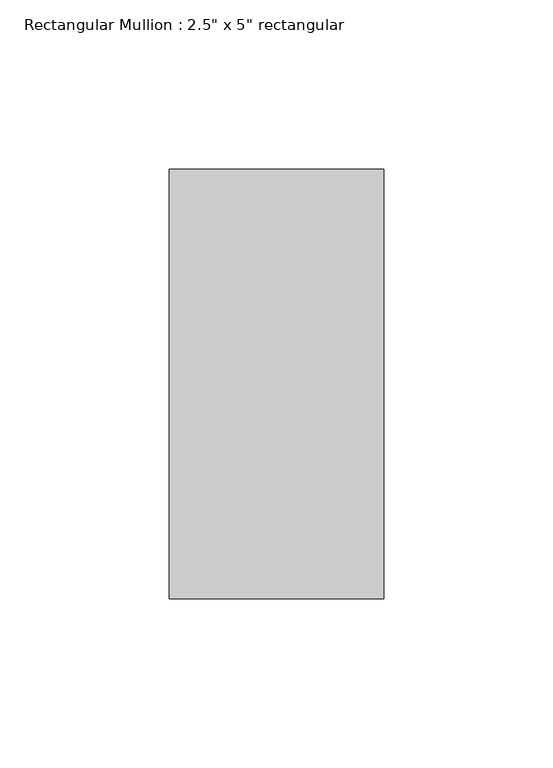
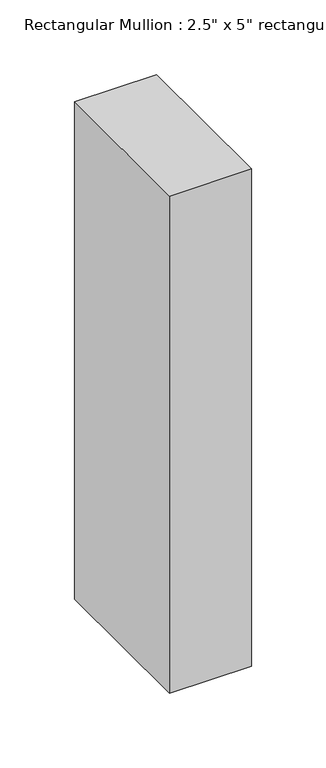
"""IFC4 building model written with IfcOpenShell, lengths in millimetres: member geometry."""

from ifc_helpers import new_model, si_unit, frame, origin, place, context, project, spatial, polyline, outline, extrude, source, transform, mapped, element, save


def member_90c805a2(model_context):
    return source(origin(), model_context, "Body", "SweptSolid", [
        extrude(outline(polyline([(31.75, 63.5), (31.75, -63.5), (-31.75, -63.5), (-31.75, 63.5), (31.75, 63.5)])), frame((0.0, 0.0, -406.4), z_axis=(0.0, 0.0, 1.0), x_axis=(1.0, 0.0, 0.0)), (0.0, 0.0, 1.0), 406.4),
    ])


if __name__ == "__main__":
    model = new_model("IFC4")
    model_context = context("Model", 3, world=origin())
    ifc_project = project(units=[si_unit("LENGTHUNIT", "METRE", prefix="MILLI")], contexts=[model_context])
    site = spatial("IfcSite", under=ifc_project)
    building = spatial("IfcBuilding", under=site)
    placement = place(None, origin())
    member_shape = member_90c805a2(model_context)
    element("IfcMember", 1, ObjectType="Rectangular Mullion : 2.5\" x 5\" rectangular", at=placement, inside=building, context=model_context, shape_type="MappedRepresentation", body=[
        mapped(member_shape, transform((0.0, 0.0, 0.0), x_axis=(1.0, 0.0, 0.0), y_axis=(0.0, 1.0, 0.0), z_axis=(0.0, 0.0, 1.0))),
    ])
    save(model, "model.ifc")

# Revit data of these elements
# Type "Rectangular Mullion : 2.5\" x 5\" rectangular"
#   built-in parameter 1007304 = 0.416667 (stored number, unit not read)
#   built-in parameter 1007301 = 0.104167 (stored number, unit not read)
#   built-in parameter 1007300 = 0.104167 (stored number, unit not read)
